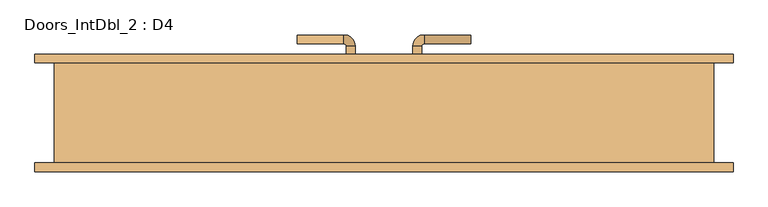
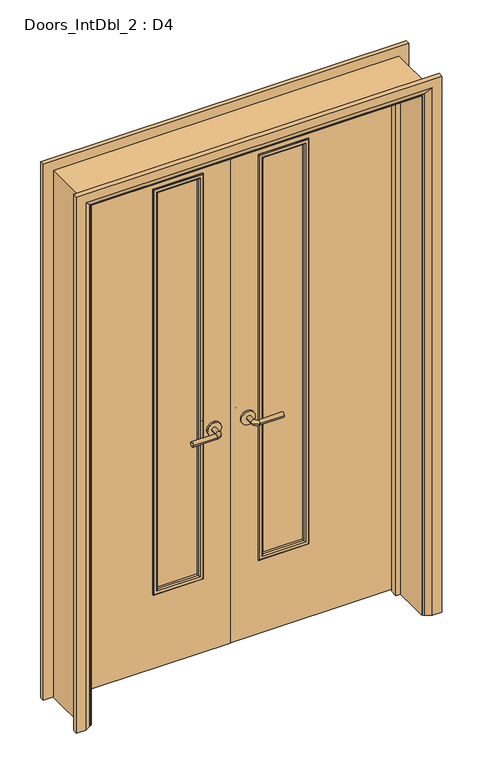
"""IFC4 building model written with IfcOpenShell, lengths in millimetres: door geometry, Doors_IntDbl_2 : D4."""

from ifc_helpers import new_model, si_unit, point, frame, frame_2d, origin, place, context, project, spatial, polyline, circle_curve, ellipse_curve, trimmed, segment, composite_curve, outline, extrude, faceted_brep, source, transform, mapped, element, save
from ifc_brep_helpers import plane_surface, cylinder_surface, revolved_surface, advanced_brep


def doors_intdbl_2_d4_7d0a9876(model_context):
    return source(origin(), model_context, "Body", "SolidModel", [
        advanced_brep(
        [(-65.0, 72.5, 1007.0), (-85.0, 72.5, 1007.0), (-65.0, 42.5, 1007.0), (-85.0, 42.5, 1007.0), (-90.0, 37.5, 1007.0), (-90.0, 17.5, 1007.0), (-195.0, 17.5, 1007.0), (-195.0, 37.5, 1007.0)],
        [
            (0, 1, circle_curve(frame((-75.0, 72.5, 1007.0), z_axis=(0.0, 1.0, 0.0), x_axis=(-1.0, 0.0, 0.0)), 10.0)),
            (1, 0, circle_curve(frame((-75.0, 72.5, 1007.0), z_axis=(0.0, 1.0, 0.0), x_axis=(-1.0, 0.0, 0.0)), 10.0)),
            (0, 2),
            (2, 3, circle_curve(frame((-75.0, 42.5, 1007.0), z_axis=(0.0, 1.0, 0.0), x_axis=(-1.0, 0.0, 0.0)), 10.0)),
            (3, 1),
            (3, 2, circle_curve(frame((-75.0, 42.5, 1007.0), z_axis=(0.0, 1.0, 0.0), x_axis=(-1.0, 0.0, 0.0)), 10.0)),
            (4, 3, circle_curve(frame((-90.0, 42.5, 1007.0), z_axis=(0.0, 0.0, 1.0), x_axis=(1.0, 0.0, 0.0)), 5.0)),
            (2, 5, circle_curve(frame((-90.0, 42.5, 1007.0), z_axis=(0.0, 0.0, -1.0), x_axis=(1.0, 0.0, 0.0)), 25.0)),
            (5, 4, circle_curve(frame((-90.0, 27.5, 1007.0), z_axis=(1.0, 0.0, 0.0), x_axis=(0.0, 1.0, 0.0)), 10.0)),
            (4, 5, circle_curve(frame((-90.0, 27.5, 1007.0), z_axis=(1.0, 0.0, 0.0), x_axis=(0.0, 1.0, 0.0)), 10.0)),
            (6, 7, circle_curve(frame((-195.0, 27.5, 1007.0), z_axis=(-1.0, 0.0, 0.0), x_axis=(0.0, 1.0, 0.0)), 10.0)),
            (7, 6, circle_curve(frame((-195.0, 27.5, 1007.0), z_axis=(-1.0, 0.0, 0.0), x_axis=(0.0, 1.0, 0.0)), 10.0)),
            (5, 6),
            (7, 4),
        ],
        [
            plane_surface(frame((-75.0, 72.5, 1007.0), z_axis=(0.0, 1.0, 0.0), x_axis=(0.0, 0.0, 1.0))),
            cylinder_surface(frame((-75.0, 72.5, 1007.0), z_axis=(0.0, 1.0, 0.0), x_axis=(-1.0, 0.0, 0.0)), 10.0),
            revolved_surface(trimmed(ellipse_curve(frame((-75.0, 42.5, 1007.0), z_axis=(0.0, 1.0, 0.0), x_axis=(-1.0, 0.0, 0.0)), 10.0, 10.0), [point((-65.0, 42.5, 1007.0))], [point((-85.0, 42.5, 1007.0))], True, "CARTESIAN"), (-90.0, 42.5, 1007.0), (0.0, 0.0, -1.0)),
            revolved_surface(trimmed(ellipse_curve(frame((-75.0, 42.5, 1007.0), z_axis=(0.0, 1.0, 0.0), x_axis=(-1.0, 0.0, 0.0)), 10.0, 10.0), [point((-85.0, 42.5, 1007.0))], [point((-65.0, 42.5, 1007.0))], True, "CARTESIAN"), (-90.0, 42.5, 1007.0), (0.0, 0.0, -1.0)),
            plane_surface(frame((-195.0, 27.5, 1007.0), z_axis=(-1.0, 0.0, 0.0), x_axis=(0.0, 0.0, 1.0))),
            cylinder_surface(frame((-90.0, 27.5, 1007.0), z_axis=(1.0, 0.0, 0.0), x_axis=(0.0, 1.0, 0.0)), 10.0),
        ],
        [
            (0, [[1, 2]]),
            (1, [[-1, 3, 4, 5]]),
            (1, [[-2, -5, 6, -3]]),
            (2, [[7, -4, 8, 9]]),
            (3, [[-8, -6, -7, 10]]),
            (4, [[11, 12]]),
            (5, [[-9, 13, -12, 14]]),
            (5, [[-10, -14, -11, -13]]),
        ],
    ),
        extrude(outline(composite_curve([segment(trimmed(circle_curve(frame_2d((1007.0, -72.5)), 30.0), [point((1007.0, -42.5))], [point((1007.0, -102.5))], False, "CARTESIAN"), True, "CONTINUOUS"), segment(trimmed(circle_curve(frame_2d((1007.0, -72.5)), 30.0), [point((1007.0, -102.5))], [point((1007.0, -42.5))], False, "CARTESIAN"), True, "CONTINUOUS")], self_intersect=False)), frame((0.0, 72.5, 0.0), z_axis=(0.0, 1.0, 0.0), x_axis=(0.0, 0.0, 1.0)), (0.0, 0.0, 1.0), 8.0),
        advanced_brep(
        [(-65.0, 120.5, 1007.0), (-85.0, 120.5, 1007.0), (-85.0, 150.5, 1007.0), (-65.0, 150.5, 1007.0), (-90.0, 155.5, 1007.0), (-90.0, 175.5, 1007.0), (-195.0, 175.5, 1007.0), (-195.0, 155.5, 1007.0)],
        [
            (0, 1, circle_curve(frame((-75.0, 120.5, 1007.0), z_axis=(0.0, -1.0, 0.0), x_axis=(-1.0, 0.0, 0.0)), 10.0)),
            (1, 0, circle_curve(frame((-75.0, 120.5, 1007.0), z_axis=(0.0, -1.0, 0.0), x_axis=(-1.0, 0.0, 0.0)), 10.0)),
            (1, 2),
            (2, 3, circle_curve(frame((-75.0, 150.5, 1007.0), z_axis=(0.0, -1.0, 0.0), x_axis=(-1.0, 0.0, 0.0)), 10.0)),
            (3, 0),
            (3, 2, circle_curve(frame((-75.0, 150.5, 1007.0), z_axis=(0.0, -1.0, 0.0), x_axis=(-1.0, 0.0, 0.0)), 10.0)),
            (4, 5, circle_curve(frame((-90.0, 165.5, 1007.0), z_axis=(1.0, 0.0, 0.0), x_axis=(0.0, -1.0, 0.0)), 10.0)),
            (5, 3, circle_curve(frame((-90.0, 150.5, 1007.0), z_axis=(0.0, 0.0, -1.0), x_axis=(1.0, 0.0, 0.0)), 25.0)),
            (2, 4, circle_curve(frame((-90.0, 150.5, 1007.0), z_axis=(0.0, 0.0, 1.0), x_axis=(1.0, 0.0, 0.0)), 5.0)),
            (5, 4, circle_curve(frame((-90.0, 165.5, 1007.0), z_axis=(1.0, 0.0, 0.0), x_axis=(0.0, -1.0, 0.0)), 10.0)),
            (6, 7, circle_curve(frame((-195.0, 165.5, 1007.0), z_axis=(-1.0, 0.0, 0.0), x_axis=(0.0, -1.0, 0.0)), 10.0)),
            (7, 6, circle_curve(frame((-195.0, 165.5, 1007.0), z_axis=(-1.0, 0.0, 0.0), x_axis=(0.0, -1.0, 0.0)), 10.0)),
            (4, 7),
            (6, 5),
        ],
        [
            plane_surface(frame((-75.0, 120.5, 1007.0), z_axis=(0.0, -1.0, 0.0), x_axis=(0.0, 0.0, 1.0))),
            cylinder_surface(frame((-75.0, 120.5, 1007.0), z_axis=(0.0, -1.0, 0.0), x_axis=(-1.0, 0.0, 0.0)), 10.0),
            revolved_surface(trimmed(ellipse_curve(frame((-75.0, 150.5, 1007.0), z_axis=(0.0, 1.0, 0.0), x_axis=(-1.0, 0.0, 0.0)), 10.0, 10.0), [point((-65.0, 150.5, 1007.0))], [point((-85.0, 150.5, 1007.0))], True, "CARTESIAN"), (-90.0, 150.5, 1007.0), (0.0, 0.0, -1.0)),
            revolved_surface(trimmed(ellipse_curve(frame((-75.0, 150.5, 1007.0), z_axis=(0.0, 1.0, 0.0), x_axis=(-1.0, 0.0, 0.0)), 10.0, 10.0), [point((-85.0, 150.5, 1007.0))], [point((-65.0, 150.5, 1007.0))], True, "CARTESIAN"), (-90.0, 150.5, 1007.0), (0.0, 0.0, -1.0)),
            plane_surface(frame((-195.0, 165.5, 1007.0), z_axis=(-1.0, 0.0, 0.0), x_axis=(0.0, 0.0, 1.0))),
            cylinder_surface(frame((-90.0, 165.5, 1007.0), z_axis=(1.0, 0.0, 0.0), x_axis=(0.0, -1.0, 0.0)), 10.0),
        ],
        [
            (0, [[1, 2]]),
            (1, [[3, 4, 5, -2]]),
            (1, [[-5, 6, -3, -1]]),
            (2, [[7, 8, -4, 9]]),
            (3, [[10, -9, -6, -8]]),
            (4, [[11, 12]]),
            (5, [[13, -11, 14, -7]]),
            (5, [[-14, -12, -13, -10]]),
        ],
    ),
        extrude(outline(composite_curve([segment(trimmed(circle_curve(frame_2d((1007.0, -72.5)), 30.0), [point((1007.0, -42.5))], [point((1007.0, -102.5))], False, "CARTESIAN"), True, "CONTINUOUS"), segment(trimmed(circle_curve(frame_2d((1007.0, -72.5)), 30.0), [point((1007.0, -102.5))], [point((1007.0, -42.5))], False, "CARTESIAN"), True, "CONTINUOUS")], self_intersect=False)), frame((0.0, 112.5, 0.0), z_axis=(0.0, 1.0, 0.0), x_axis=(0.0, 0.0, 1.0)), (0.0, 0.0, 1.0), 8.0),
        advanced_brep(
        [(65.0, 72.5, 1007.0), (85.0, 72.5, 1007.0), (85.0, 42.5, 1007.0), (65.0, 42.5, 1007.0), (90.0, 37.5, 1007.0), (90.0, 17.5, 1007.0), (195.0, 17.5, 1007.0), (195.0, 37.5, 1007.0)],
        [
            (0, 1, circle_curve(frame((75.0, 72.5, 1007.0), z_axis=(0.0, 1.0, 0.0), x_axis=(1.0, 0.0, 0.0)), 10.0)),
            (1, 0, circle_curve(frame((75.0, 72.5, 1007.0), z_axis=(0.0, 1.0, 0.0), x_axis=(1.0, 0.0, 0.0)), 10.0)),
            (1, 2),
            (2, 3, circle_curve(frame((75.0, 42.5, 1007.0), z_axis=(0.0, 1.0, 0.0), x_axis=(1.0, 0.0, 0.0)), 10.0)),
            (3, 0),
            (3, 2, circle_curve(frame((75.0, 42.5, 1007.0), z_axis=(0.0, 1.0, 0.0), x_axis=(1.0, 0.0, 0.0)), 10.0)),
            (4, 5, circle_curve(frame((90.0, 27.5, 1007.0), z_axis=(-1.0, 0.0, 0.0), x_axis=(0.0, 1.0, 0.0)), 10.0)),
            (5, 3, circle_curve(frame((90.0, 42.5, 1007.0), z_axis=(0.0, 0.0, -1.0), x_axis=(-1.0, 0.0, 0.0)), 25.0)),
            (2, 4, circle_curve(frame((90.0, 42.5, 1007.0), z_axis=(0.0, 0.0, 1.0), x_axis=(-1.0, 0.0, 0.0)), 5.0)),
            (5, 4, circle_curve(frame((90.0, 27.5, 1007.0), z_axis=(-1.0, 0.0, 0.0), x_axis=(0.0, 1.0, 0.0)), 10.0)),
            (6, 7, circle_curve(frame((195.0, 27.5, 1007.0), z_axis=(1.0, 0.0, 0.0), x_axis=(0.0, 1.0, 0.0)), 10.0)),
            (7, 6, circle_curve(frame((195.0, 27.5, 1007.0), z_axis=(1.0, 0.0, 0.0), x_axis=(0.0, 1.0, 0.0)), 10.0)),
            (4, 7),
            (6, 5),
        ],
        [
            plane_surface(frame((75.0, 72.5, 1007.0), z_axis=(0.0, 1.0, 0.0), x_axis=(0.0, 0.0, 1.0))),
            cylinder_surface(frame((75.0, 72.5, 1007.0), z_axis=(0.0, 1.0, 0.0), x_axis=(1.0, 0.0, 0.0)), 10.0),
            revolved_surface(trimmed(ellipse_curve(frame((75.0, 42.5, 1007.0), z_axis=(0.0, -1.0, 0.0), x_axis=(1.0, 0.0, 0.0)), 10.0, 10.0), [point((65.0, 42.5, 1007.0))], [point((85.0, 42.5, 1007.0))], True, "CARTESIAN"), (90.0, 42.5, 1007.0), (0.0, 0.0, -1.0)),
            revolved_surface(trimmed(ellipse_curve(frame((75.0, 42.5, 1007.0), z_axis=(0.0, -1.0, 0.0), x_axis=(1.0, 0.0, 0.0)), 10.0, 10.0), [point((85.0, 42.5, 1007.0))], [point((65.0, 42.5, 1007.0))], True, "CARTESIAN"), (90.0, 42.5, 1007.0), (0.0, 0.0, -1.0)),
            plane_surface(frame((195.0, 27.5, 1007.0), z_axis=(1.0, 0.0, 0.0), x_axis=(0.0, 0.0, 1.0))),
            cylinder_surface(frame((90.0, 27.5, 1007.0), z_axis=(-1.0, 0.0, 0.0), x_axis=(0.0, 1.0, 0.0)), 10.0),
        ],
        [
            (0, [[1, 2]]),
            (1, [[3, 4, 5, -2]]),
            (1, [[-5, 6, -3, -1]]),
            (2, [[7, 8, -4, 9]]),
            (3, [[10, -9, -6, -8]]),
            (4, [[11, 12]]),
            (5, [[13, -11, 14, -7]]),
            (5, [[-14, -12, -13, -10]]),
        ],
    ),
        extrude(outline(composite_curve([segment(trimmed(circle_curve(frame_2d((1007.0, 72.5)), 30.0), [point((1007.0, 42.5))], [point((1007.0, 102.5))], False, "CARTESIAN"), True, "CONTINUOUS"), segment(trimmed(circle_curve(frame_2d((1007.0, 72.5)), 30.0), [point((1007.0, 102.5))], [point((1007.0, 42.5))], False, "CARTESIAN"), True, "CONTINUOUS")], self_intersect=False)), frame((0.0, 72.5, 0.0), z_axis=(0.0, 1.0, 0.0), x_axis=(0.0, 0.0, 1.0)), (0.0, 0.0, 1.0), 8.0),
        advanced_brep(
        [(65.0, 120.5, 1007.0), (85.0, 120.5, 1007.0), (65.0, 150.5, 1007.0), (85.0, 150.5, 1007.0), (90.0, 155.5, 1007.0), (90.0, 175.5, 1007.0), (195.0, 175.5, 1007.0), (195.0, 155.5, 1007.0)],
        [
            (0, 1, circle_curve(frame((75.0, 120.5, 1007.0), z_axis=(0.0, -1.0, 0.0), x_axis=(1.0, 0.0, 0.0)), 10.0)),
            (1, 0, circle_curve(frame((75.0, 120.5, 1007.0), z_axis=(0.0, -1.0, 0.0), x_axis=(1.0, 0.0, 0.0)), 10.0)),
            (0, 2),
            (2, 3, circle_curve(frame((75.0, 150.5, 1007.0), z_axis=(0.0, -1.0, 0.0), x_axis=(1.0, 0.0, 0.0)), 10.0)),
            (3, 1),
            (3, 2, circle_curve(frame((75.0, 150.5, 1007.0), z_axis=(0.0, -1.0, 0.0), x_axis=(1.0, 0.0, 0.0)), 10.0)),
            (4, 3, circle_curve(frame((90.0, 150.5, 1007.0), z_axis=(0.0, 0.0, 1.0), x_axis=(-1.0, 0.0, 0.0)), 5.0)),
            (2, 5, circle_curve(frame((90.0, 150.5, 1007.0), z_axis=(0.0, 0.0, -1.0), x_axis=(-1.0, 0.0, 0.0)), 25.0)),
            (5, 4, circle_curve(frame((90.0, 165.5, 1007.0), z_axis=(-1.0, 0.0, 0.0), x_axis=(0.0, -1.0, 0.0)), 10.0)),
            (4, 5, circle_curve(frame((90.0, 165.5, 1007.0), z_axis=(-1.0, 0.0, 0.0), x_axis=(0.0, -1.0, 0.0)), 10.0)),
            (6, 7, circle_curve(frame((195.0, 165.5, 1007.0), z_axis=(1.0, 0.0, 0.0), x_axis=(0.0, -1.0, 0.0)), 10.0)),
            (7, 6, circle_curve(frame((195.0, 165.5, 1007.0), z_axis=(1.0, 0.0, 0.0), x_axis=(0.0, -1.0, 0.0)), 10.0)),
            (5, 6),
            (7, 4),
        ],
        [
            plane_surface(frame((75.0, 120.5, 1007.0), z_axis=(0.0, -1.0, 0.0), x_axis=(0.0, 0.0, 1.0))),
            cylinder_surface(frame((75.0, 120.5, 1007.0), z_axis=(0.0, -1.0, 0.0), x_axis=(1.0, 0.0, 0.0)), 10.0),
            revolved_surface(trimmed(ellipse_curve(frame((75.0, 150.5, 1007.0), z_axis=(0.0, -1.0, 0.0), x_axis=(1.0, 0.0, 0.0)), 10.0, 10.0), [point((65.0, 150.5, 1007.0))], [point((85.0, 150.5, 1007.0))], True, "CARTESIAN"), (90.0, 150.5, 1007.0), (0.0, 0.0, -1.0)),
            revolved_surface(trimmed(ellipse_curve(frame((75.0, 150.5, 1007.0), z_axis=(0.0, -1.0, 0.0), x_axis=(1.0, 0.0, 0.0)), 10.0, 10.0), [point((85.0, 150.5, 1007.0))], [point((65.0, 150.5, 1007.0))], True, "CARTESIAN"), (90.0, 150.5, 1007.0), (0.0, 0.0, -1.0)),
            plane_surface(frame((195.0, 165.5, 1007.0), z_axis=(1.0, 0.0, 0.0), x_axis=(0.0, 0.0, 1.0))),
            cylinder_surface(frame((90.0, 165.5, 1007.0), z_axis=(-1.0, 0.0, 0.0), x_axis=(0.0, -1.0, 0.0)), 10.0),
        ],
        [
            (0, [[1, 2]]),
            (1, [[-1, 3, 4, 5]]),
            (1, [[-2, -5, 6, -3]]),
            (2, [[7, -4, 8, 9]]),
            (3, [[-8, -6, -7, 10]]),
            (4, [[11, 12]]),
            (5, [[-9, 13, -12, 14]]),
            (5, [[-10, -14, -11, -13]]),
        ],
    ),
        extrude(outline(composite_curve([segment(trimmed(circle_curve(frame_2d((1007.0, 72.5)), 30.0), [point((1007.0, 42.5))], [point((1007.0, 102.5))], False, "CARTESIAN"), True, "CONTINUOUS"), segment(trimmed(circle_curve(frame_2d((1007.0, 72.5)), 30.0), [point((1007.0, 102.5))], [point((1007.0, 42.5))], False, "CARTESIAN"), True, "CONTINUOUS")], self_intersect=False)), frame((0.0, 112.5, 0.0), z_axis=(0.0, 1.0, 0.0), x_axis=(0.0, 0.0, 1.0)), (0.0, 0.0, 1.0), 8.0),
        extrude(outline(polyline([(2392.0, -742.0), (0.0, -742.0), (0.0, -710.0), (2360.0, -710.0), (2360.0, 710.0), (0.0, 710.0), (0.0, 742.0), (2392.0, 742.0), (2392.0, -742.0)])), frame((0.0, -112.5, 0.0), z_axis=(0.0, 1.0, 0.0), x_axis=(0.0, 0.0, 1.0)), (0.0, 0.0, 1.0), 225.0),
        faceted_brep([(-691.0, 77.5, 0.0), (-691.0, 45.5, 0.0), (-710.0, 45.5, 0.0), (-710.0, 77.5, 0.0), (-691.0, 77.5, 2341.0), (-691.0, 45.5, 2341.0), (-710.0, 45.5, 2360.0), (-710.0, 77.5, 2360.0), (691.0, 77.5, 0.0), (710.0, 77.5, 0.0), (710.0, 45.5, 0.0), (691.0, 45.5, 0.0), (691.0, 77.5, 2341.0), (710.0, 77.5, 2360.0), (710.0, 45.5, 2360.0), (691.0, 45.5, 2341.0)], [[[0, 1, 2, 3]], [[1, 0, 4, 5]], [[2, 1, 5, 6]], [[3, 2, 6, 7]], [[0, 3, 7, 4]], [[8, 9, 10, 11]], [[12, 13, 9, 8]], [[13, 14, 10, 9]], [[14, 15, 11, 10]], [[15, 12, 8, 11]], [[5, 4, 12, 15]], [[6, 5, 15, 14]], [[7, 6, 14, 13]], [[4, 7, 13, 12]]]),
        advanced_brep(
        [(785.0, 132.5, 0.0), (785.0, 112.5, 0.0), (715.0, 112.5, 0.0), (719.0, 118.5, 0.0), (745.0, 132.5, 0.0), (785.0, 132.5, 2435.0), (785.0, 112.5, 2435.0), (-785.0, 112.5, 2435.0), (-785.0, 112.5, 0.0), (-715.0, 112.5, 0.0), (-715.0, 112.5, 2365.0), (715.0, 112.5, 2365.0), (719.0, 118.5, 2369.0), (745.0, 132.5, 2395.0), (-745.0, 132.5, 2395.0), (-745.0, 132.5, 0.0), (-785.0, 132.5, 0.0), (-785.0, 132.5, 2435.0), (-719.0, 118.5, 0.0), (-719.0, 118.5, 2369.0)],
        [
            (0, 1),
            (1, 2),
            (2, 3, circle_curve(frame((723.0, 111.5, 0.0), z_axis=(0.0, 0.0, -1.0), x_axis=(1.0, 0.0, 0.0)), 8.0622577)),
            (3, 4),
            (4, 0),
            (0, 5),
            (5, 6),
            (6, 1),
            (6, 7),
            (7, 8),
            (8, 9),
            (9, 10),
            (10, 11),
            (11, 2),
            (11, 12, ellipse_curve(frame((723.0, 111.5, 2373.0), z_axis=(0.7071067811865475, 0.0, -0.7071067811865475), x_axis=(-0.7071067811865474, 0.0, -0.7071067811865476)), 11.4017543, 8.0622577)),
            (12, 3),
            (12, 13),
            (13, 4),
            (13, 14),
            (14, 15),
            (15, 16),
            (16, 17),
            (17, 5),
            (7, 17),
            (16, 8),
            (15, 18),
            (18, 9, circle_curve(frame((-723.0, 111.5, 0.0), z_axis=(0.0, 0.0, -1.0), x_axis=(-1.0, 0.0, 0.0)), 8.0622577)),
            (19, 10, ellipse_curve(frame((-723.0, 111.5, 2373.0), z_axis=(-0.7071067811865475, 0.0, -0.7071067811865475), x_axis=(-0.7071067811865474, 0.0, 0.7071067811865476)), 11.4017543, 8.0622577)),
            (18, 19),
            (14, 19),
            (19, 12),
        ],
        [
            plane_surface(frame((715.0, 112.5, 0.0), z_axis=(0.0, 0.0, -1.0), x_axis=(0.0, -1.0, 0.0))),
            plane_surface(frame((785.0, 132.5, 0.0), z_axis=(1.0, 0.0, 0.0), x_axis=(0.0, 0.0, 1.0))),
            plane_surface(frame((785.0, 112.5, 0.0), z_axis=(0.0, -1.0, 0.0), x_axis=(0.0, 0.0, 1.0))),
            cylinder_surface(frame((723.0, 111.5, 0.0), z_axis=(0.0, 0.0, -1.0), x_axis=(1.0, 0.0, 0.0)), 8.0622577),
            plane_surface(frame((719.0, 118.5, 0.0), z_axis=(-0.4740998230350126, 0.8804710999221779, 0.0), x_axis=(0.0, 0.0, 1.0))),
            plane_surface(frame((745.0, 132.5, 0.0), z_axis=(0.0, 1.0, 0.0), x_axis=(0.0, 0.0, 1.0))),
            plane_surface(frame((-785.0, 132.5, 2435.0), z_axis=(-1.0, 0.0, 0.0), x_axis=(0.0, 0.0, -1.0))),
            plane_surface(frame((-715.0, 112.5, 0.0), z_axis=(0.0, 0.0, -1.0), x_axis=(0.0, -1.0, 0.0))),
            cylinder_surface(frame((-723.0, 111.5, 2365.0), z_axis=(0.0, 0.0, 1.0), x_axis=(-1.0, 0.0, 0.0)), 8.0622577),
            plane_surface(frame((-719.0, 118.5, 2369.0), z_axis=(0.4740998230350183, 0.8804710999221749, 0.0), x_axis=(0.0, 0.0, -1.0))),
            plane_surface(frame((785.0, 132.5, 2435.0), z_axis=(0.0, 0.0, 1.0), x_axis=(-1.0, 0.0, 0.0))),
            cylinder_surface(frame((715.0, 111.5, 2373.0), z_axis=(1.0, 0.0, 0.0), x_axis=(0.0, 0.0, 1.0)), 8.0622577),
            plane_surface(frame((719.0, 118.5, 2369.0), z_axis=(0.0, 0.8804710999221763, -0.4740998230350154), x_axis=(-1.0, 0.0, 0.0))),
        ],
        [
            (0, [[1, 2, 3, 4, 5]]),
            (1, [[-1, 6, 7, 8]]),
            (2, [[-2, -8, 9, 10, 11, 12, 13, 14]]),
            (3, [[-3, -14, 15, 16]]),
            (4, [[-4, -16, 17, 18]]),
            (5, [[-5, -18, 19, 20, 21, 22, 23, -6]]),
            (6, [[24, -22, 25, -10]]),
            (7, [[-21, 26, 27, -11, -25]]),
            (8, [[28, -12, -27, 29]]),
            (9, [[30, -29, -26, -20]]),
            (10, [[-7, -23, -24, -9]]),
            (11, [[-15, -13, -28, 31]]),
            (12, [[-17, -31, -30, -19]]),
        ],
    ),
        advanced_brep(
        [(-785.0, -132.5, 0.0), (-785.0, -112.5, 0.0), (-715.0, -112.5, 0.0), (-719.0, -118.5, 0.0), (-745.0, -132.5, 0.0), (-785.0, -132.5, 2435.0), (-785.0, -112.5, 2435.0), (785.0, -112.5, 2435.0), (785.0, -112.5, 0.0), (715.0, -112.5, 0.0), (715.0, -112.5, 2365.0), (-715.0, -112.5, 2365.0), (-719.0, -118.5, 2369.0), (-745.0, -132.5, 2395.0), (745.0, -132.5, 2395.0), (745.0, -132.5, 0.0), (785.0, -132.5, 0.0), (785.0, -132.5, 2435.0), (719.0, -118.5, 0.0), (719.0, -118.5, 2369.0)],
        [
            (0, 1),
            (1, 2),
            (2, 3, circle_curve(frame((-723.0, -111.5, 0.0), z_axis=(0.0, 0.0, -1.0), x_axis=(-1.0, 0.0, 0.0)), 8.0622577)),
            (3, 4),
            (4, 0),
            (0, 5),
            (5, 6),
            (6, 1),
            (6, 7),
            (7, 8),
            (8, 9),
            (9, 10),
            (10, 11),
            (11, 2),
            (11, 12, ellipse_curve(frame((-723.0, -111.5, 2373.0), z_axis=(-0.7071067811865475, 0.0, -0.7071067811865475), x_axis=(0.7071067811865474, 0.0, -0.7071067811865476)), 11.4017543, 8.0622577)),
            (12, 3),
            (12, 13),
            (13, 4),
            (13, 14),
            (14, 15),
            (15, 16),
            (16, 17),
            (17, 5),
            (7, 17),
            (16, 8),
            (15, 18),
            (18, 9, circle_curve(frame((723.0, -111.5, 0.0), z_axis=(0.0, 0.0, -1.0), x_axis=(1.0, 0.0, 0.0)), 8.0622577)),
            (19, 10, ellipse_curve(frame((723.0, -111.5, 2373.0), z_axis=(0.7071067811865475, 0.0, -0.7071067811865475), x_axis=(0.7071067811865474, 0.0, 0.7071067811865476)), 11.4017543, 8.0622577)),
            (18, 19),
            (14, 19),
            (19, 12),
        ],
        [
            plane_surface(frame((-715.0, -112.5, 0.0), z_axis=(0.0, 0.0, -1.0), x_axis=(0.0, -1.0, 0.0))),
            plane_surface(frame((-785.0, -132.5, 0.0), z_axis=(-1.0, 0.0, 0.0), x_axis=(0.0, 0.0, 1.0))),
            plane_surface(frame((-785.0, -112.5, 0.0), z_axis=(0.0, 1.0, 0.0), x_axis=(0.0, 0.0, 1.0))),
            cylinder_surface(frame((-723.0, -111.5, 0.0), z_axis=(0.0, 0.0, -1.0), x_axis=(-1.0, 0.0, 0.0)), 8.0622577),
            plane_surface(frame((-719.0, -118.5, 0.0), z_axis=(0.4740998230350183, -0.8804710999221749, 0.0), x_axis=(0.0, 0.0, 1.0))),
            plane_surface(frame((-745.0, -132.5, 0.0), z_axis=(0.0, -1.0, 0.0), x_axis=(0.0, 0.0, 1.0))),
            plane_surface(frame((785.0, -132.5, 2435.0), z_axis=(1.0, 0.0, 0.0), x_axis=(0.0, 0.0, -1.0))),
            plane_surface(frame((715.0, -112.5, 0.0), z_axis=(0.0, 0.0, -1.0), x_axis=(0.0, -1.0, 0.0))),
            cylinder_surface(frame((723.0, -111.5, 2365.0), z_axis=(0.0, 0.0, 1.0), x_axis=(1.0, 0.0, 0.0)), 8.0622577),
            plane_surface(frame((719.0, -118.5, 2369.0), z_axis=(-0.4740998230350183, -0.8804710999221749, 0.0), x_axis=(0.0, 0.0, -1.0))),
            plane_surface(frame((-785.0, -132.5, 2435.0), z_axis=(0.0, 0.0, 1.0), x_axis=(1.0, 0.0, 0.0))),
            cylinder_surface(frame((-715.0, -111.5, 2373.0), z_axis=(-1.0, 0.0, 0.0), x_axis=(0.0, 0.0, 1.0)), 8.0622577),
            plane_surface(frame((-719.0, -118.5, 2369.0), z_axis=(0.0, -0.8804710999221749, -0.4740998230350183), x_axis=(1.0, 0.0, 0.0))),
        ],
        [
            (0, [[1, 2, 3, 4, 5]]),
            (1, [[-1, 6, 7, 8]]),
            (2, [[-2, -8, 9, 10, 11, 12, 13, 14]]),
            (3, [[-3, -14, 15, 16]]),
            (4, [[-4, -16, 17, 18]]),
            (5, [[-5, -18, 19, 20, 21, 22, 23, -6]]),
            (6, [[24, -22, 25, -10]]),
            (7, [[-21, 26, 27, -11, -25]]),
            (8, [[28, -12, -27, 29]]),
            (9, [[30, -29, -26, -20]]),
            (10, [[-7, -23, -24, -9]]),
            (11, [[-15, -13, -28, 31]]),
            (12, [[-17, -31, -30, -19]]),
        ],
    ),
        extrude(outline(polyline([(5.753223, 707.0), (2357.0, 707.0), (2357.0, 1.5), (5.753223, 1.5), (5.753223, 707.0)]), holes=[polyline([(2175.0, 126.5), (2175.0, 326.5), (350.0, 326.5), (350.0, 126.5), (2175.0, 126.5)])]), frame((0.0, 80.5, 0.0), z_axis=(0.0, 1.0, 0.0), x_axis=(0.0, 0.0, 1.0)), (0.0, 0.0, 1.0), 32.0),
        extrude(outline(polyline([(5.753223, -707.0), (5.753223, -1.5), (2357.0, -1.5), (2357.0, -707.0), (5.753223, -707.0)]), holes=[polyline([(2175.0, -326.5), (2175.0, -126.5), (350.0, -126.5), (350.0, -326.5), (2175.0, -326.5)])]), frame((0.0, 80.5, 0.0), z_axis=(0.0, 1.0, 0.0), x_axis=(0.0, 0.0, 1.0)), (0.0, 0.0, 1.0), 32.0),
        extrude(outline(polyline([(326.5, 90.5), (126.5, 90.5), (126.5, 102.5), (326.5, 102.5), (326.5, 90.5)])), frame((0.0, 0.0, 350.0), z_axis=(0.0, 0.0, 1.0), x_axis=(1.0, 0.0, 0.0)), (0.0, 0.0, 1.0), 1825.0),
        extrude(outline(polyline([(-126.5, 90.5), (-326.5, 90.5), (-326.5, 102.5), (-126.5, 102.5), (-126.5, 90.5)])), frame((0.0, 0.0, 350.0), z_axis=(0.0, 0.0, 1.0), x_axis=(1.0, 0.0, 0.0)), (0.0, 0.0, 1.0), 1825.0),
        advanced_brep(
        [(-326.5, 102.5, 2175.0), (-326.5, 112.5, 2175.0), (-326.5, 112.5, 350.0), (-326.5, 102.5, 350.0), (-314.5, 113.5, 2163.0), (-314.5, 102.5, 2163.0), (-314.5, 102.5, 362.0), (-314.5, 113.5, 362.0), (-319.5, 118.5, 2168.0), (-319.5, 118.5, 357.0), (-334.5, 116.5, 2183.0), (-332.5, 118.5, 2181.0), (-332.5, 118.5, 344.0), (-334.5, 116.5, 342.0), (-334.5, 112.5, 2183.0), (-334.5, 112.5, 342.0), (-126.5, 112.5, 350.0), (-126.5, 102.5, 350.0), (-138.5, 102.5, 362.0), (-138.5, 113.5, 362.0), (-133.5, 118.5, 357.0), (-120.5, 118.5, 344.0), (-118.5, 116.5, 342.0), (-118.5, 112.5, 342.0), (-126.5, 112.5, 2175.0), (-126.5, 102.5, 2175.0), (-138.5, 102.5, 2163.0), (-138.5, 113.5, 2163.0), (-133.5, 118.5, 2168.0), (-120.5, 118.5, 2181.0), (-118.5, 116.5, 2183.0), (-118.5, 112.5, 2183.0)],
        [
            (0, 1),
            (1, 2),
            (2, 3),
            (3, 0),
            (4, 5),
            (5, 6),
            (6, 7),
            (7, 4),
            (8, 4, ellipse_curve(frame((-319.5, 113.5, 2168.0), z_axis=(-0.7071067811865475, 0.0, -0.7071067811865475), x_axis=(-0.7071067811865474, 0.0, 0.7071067811865476)), 7.0710678, 5.0)),
            (7, 9, ellipse_curve(frame((-319.5, 113.5, 357.0), z_axis=(-0.7071067811865475, 0.0, 0.7071067811865475), x_axis=(0.7071067811865474, 0.0, 0.7071067811865476)), 7.0710678, 5.0)),
            (9, 8),
            (10, 11, ellipse_curve(frame((-332.5, 116.5, 2181.0), z_axis=(-0.7071067811865475, 0.0, -0.7071067811865475), x_axis=(-0.7071067811865474, 0.0, 0.7071067811865476)), 2.8284271, 2.0)),
            (11, 12),
            (12, 13, ellipse_curve(frame((-332.5, 116.5, 344.0), z_axis=(-0.7071067811865475, 0.0, 0.7071067811865475), x_axis=(0.7071067811865474, 0.0, 0.7071067811865476)), 2.8284271, 2.0)),
            (13, 10),
            (14, 10),
            (13, 15),
            (15, 14),
            (2, 16),
            (16, 17),
            (17, 3),
            (6, 18),
            (18, 19),
            (19, 7),
            (19, 20, ellipse_curve(frame((-133.5, 113.5, 357.0), z_axis=(-0.7071067811865475, 0.0, -0.7071067811865475), x_axis=(-0.7071067811865476, 0.0, 0.7071067811865474)), 7.0710678, 5.0)),
            (20, 9),
            (12, 21),
            (21, 22, ellipse_curve(frame((-120.5, 116.5, 344.0), z_axis=(-0.7071067811865475, 0.0, -0.7071067811865475), x_axis=(-0.7071067811865476, 0.0, 0.7071067811865474)), 2.8284271, 2.0)),
            (22, 13),
            (22, 23),
            (23, 15),
            (16, 24),
            (24, 25),
            (25, 17),
            (18, 26),
            (26, 27),
            (27, 19),
            (27, 28, ellipse_curve(frame((-133.5, 113.5, 2168.0), z_axis=(0.7071067811865475, 0.0, -0.7071067811865475), x_axis=(-0.7071067811865474, 0.0, -0.7071067811865476)), 7.0710678, 5.0)),
            (28, 20),
            (21, 29),
            (29, 30, ellipse_curve(frame((-120.5, 116.5, 2181.0), z_axis=(0.7071067811865475, 0.0, -0.7071067811865475), x_axis=(-0.7071067811865474, 0.0, -0.7071067811865476)), 2.8284271, 2.0)),
            (30, 22),
            (30, 31),
            (31, 23),
            (31, 14),
            (1, 24),
            (0, 25),
            (5, 26),
            (4, 27),
            (8, 28),
            (11, 29),
            (10, 30),
        ],
        [
            plane_surface(frame((-326.5, 112.5, 2175.0), z_axis=(-1.0, 0.0, 0.0), x_axis=(0.0, 0.0, -1.0))),
            plane_surface(frame((-314.5, 102.5, 2163.0), z_axis=(1.0, 0.0, 0.0), x_axis=(0.0, 0.0, -1.0))),
            cylinder_surface(frame((-319.5, 113.5, 2175.0), z_axis=(0.0, 0.0, 1.0), x_axis=(-1.0, 0.0, 0.0)), 5.0),
            cylinder_surface(frame((-332.5, 116.5, 2175.0), z_axis=(0.0, 0.0, 1.0), x_axis=(-1.0, 0.0, 0.0)), 2.0),
            plane_surface(frame((-334.5, 116.5, 2183.0), z_axis=(-1.0, 0.0, 0.0), x_axis=(0.0, 0.0, -1.0))),
            plane_surface(frame((-326.5, 112.5, 350.0), z_axis=(0.0, 0.0, -1.0), x_axis=(1.0, 0.0, 0.0))),
            plane_surface(frame((-314.5, 102.5, 362.0), z_axis=(0.0, 0.0, 1.0), x_axis=(1.0, 0.0, 0.0))),
            cylinder_surface(frame((-326.5, 113.5, 357.0), z_axis=(-1.0, 0.0, 0.0), x_axis=(0.0, 0.0, -1.0)), 5.0),
            cylinder_surface(frame((-326.5, 116.5, 344.0), z_axis=(-1.0, 0.0, 0.0), x_axis=(0.0, 0.0, -1.0)), 2.0),
            plane_surface(frame((-334.5, 116.5, 342.0), z_axis=(0.0, 0.0, -1.0), x_axis=(1.0, 0.0, 0.0))),
            plane_surface(frame((-126.5, 112.5, 350.0), z_axis=(1.0, 0.0, 0.0), x_axis=(0.0, 0.0, 1.0))),
            plane_surface(frame((-138.5, 102.5, 362.0), z_axis=(-1.0, 0.0, 0.0), x_axis=(0.0, 0.0, 1.0))),
            cylinder_surface(frame((-133.5, 113.5, 350.0), z_axis=(0.0, 0.0, -1.0), x_axis=(1.0, 0.0, 0.0)), 5.0),
            cylinder_surface(frame((-120.5, 116.5, 350.0), z_axis=(0.0, 0.0, -1.0), x_axis=(1.0, 0.0, 0.0)), 2.0),
            plane_surface(frame((-118.5, 116.5, 342.0), z_axis=(1.0, 0.0, 0.0), x_axis=(0.0, 0.0, 1.0))),
            plane_surface(frame((-118.5, 112.5, 2183.0), z_axis=(0.0, -1.0, 0.0), x_axis=(-1.0, 0.0, 0.0))),
            plane_surface(frame((-126.5, 112.5, 2175.0), z_axis=(0.0, 0.0, 1.0), x_axis=(-1.0, 0.0, 0.0))),
            plane_surface(frame((-126.5, 102.5, 2175.0), z_axis=(0.0, -1.0, 0.0), x_axis=(-1.0, 0.0, 0.0))),
            plane_surface(frame((-138.5, 102.5, 2163.0), z_axis=(0.0, 0.0, -1.0), x_axis=(-1.0, 0.0, 0.0))),
            cylinder_surface(frame((-126.5, 113.5, 2168.0), z_axis=(1.0, 0.0, 0.0), x_axis=(0.0, 0.0, 1.0)), 5.0),
            plane_surface(frame((-133.5, 118.5, 2168.0), z_axis=(0.0, 1.0, 0.0), x_axis=(-1.0, 0.0, 0.0))),
            cylinder_surface(frame((-126.5, 116.5, 2181.0), z_axis=(1.0, 0.0, 0.0), x_axis=(0.0, 0.0, 1.0)), 2.0),
            plane_surface(frame((-118.5, 116.5, 2183.0), z_axis=(0.0, 0.0, 1.0), x_axis=(-1.0, 0.0, 0.0))),
        ],
        [
            (0, [[1, 2, 3, 4]]),
            (1, [[5, 6, 7, 8]]),
            (2, [[9, -8, 10, 11]]),
            (3, [[12, 13, 14, 15]]),
            (4, [[16, -15, 17, 18]]),
            (5, [[-3, 19, 20, 21]]),
            (6, [[-7, 22, 23, 24]]),
            (7, [[-10, -24, 25, 26]]),
            (8, [[-14, 27, 28, 29]]),
            (9, [[-17, -29, 30, 31]]),
            (10, [[-20, 32, 33, 34]]),
            (11, [[-23, 35, 36, 37]]),
            (12, [[-25, -37, 38, 39]]),
            (13, [[-28, 40, 41, 42]]),
            (14, [[-30, -42, 43, 44]]),
            (15, [[-31, -44, 45, -18], [46, -32, -19, -2]]),
            (16, [[-33, -46, -1, 47]]),
            (17, [[-21, -34, -47, -4], [48, -35, -22, -6]]),
            (18, [[-36, -48, -5, 49]]),
            (19, [[-38, -49, -9, 50]]),
            (20, [[51, -40, -27, -13], [-26, -39, -50, -11]]),
            (21, [[-41, -51, -12, 52]]),
            (22, [[-43, -52, -16, -45]]),
        ],
    ),
        advanced_brep(
        [(326.5, 102.5, 350.0), (326.5, 112.5, 350.0), (326.5, 112.5, 2175.0), (326.5, 102.5, 2175.0), (314.5, 113.5, 362.0), (314.5, 102.5, 362.0), (314.5, 102.5, 2163.0), (314.5, 113.5, 2163.0), (319.5, 118.5, 357.0), (319.5, 118.5, 2168.0), (334.5, 116.5, 342.0), (332.5, 118.5, 344.0), (332.5, 118.5, 2181.0), (334.5, 116.5, 2183.0), (334.5, 112.5, 342.0), (334.5, 112.5, 2183.0), (126.5, 112.5, 2175.0), (126.5, 102.5, 2175.0), (138.5, 102.5, 2163.0), (138.5, 113.5, 2163.0), (133.5, 118.5, 2168.0), (120.5, 118.5, 2181.0), (118.5, 116.5, 2183.0), (118.5, 112.5, 2183.0), (126.5, 112.5, 350.0), (126.5, 102.5, 350.0), (138.5, 102.5, 362.0), (138.5, 113.5, 362.0), (133.5, 118.5, 357.0), (120.5, 118.5, 344.0), (118.5, 116.5, 342.0), (118.5, 112.5, 342.0)],
        [
            (0, 1),
            (1, 2),
            (2, 3),
            (3, 0),
            (4, 5),
            (5, 6),
            (6, 7),
            (7, 4),
            (8, 4, ellipse_curve(frame((319.5, 113.5, 357.0), z_axis=(0.7071067811865475, 0.0, 0.7071067811865475), x_axis=(0.7071067811865474, 0.0, -0.7071067811865476)), 7.0710678, 5.0)),
            (7, 9, ellipse_curve(frame((319.5, 113.5, 2168.0), z_axis=(0.7071067811865475, 0.0, -0.7071067811865475), x_axis=(-0.7071067811865474, 0.0, -0.7071067811865476)), 7.0710678, 5.0)),
            (9, 8),
            (10, 11, ellipse_curve(frame((332.5, 116.5, 344.0), z_axis=(0.7071067811865475, 0.0, 0.7071067811865475), x_axis=(0.7071067811865474, 0.0, -0.7071067811865476)), 2.8284271, 2.0)),
            (11, 12),
            (12, 13, ellipse_curve(frame((332.5, 116.5, 2181.0), z_axis=(0.7071067811865475, 0.0, -0.7071067811865475), x_axis=(-0.7071067811865474, 0.0, -0.7071067811865476)), 2.8284271, 2.0)),
            (13, 10),
            (14, 10),
            (13, 15),
            (15, 14),
            (2, 16),
            (16, 17),
            (17, 3),
            (6, 18),
            (18, 19),
            (19, 7),
            (19, 20, ellipse_curve(frame((133.5, 113.5, 2168.0), z_axis=(0.7071067811865475, 0.0, 0.7071067811865475), x_axis=(0.7071067811865476, 0.0, -0.7071067811865474)), 7.0710678, 5.0)),
            (20, 9),
            (12, 21),
            (21, 22, ellipse_curve(frame((120.5, 116.5, 2181.0), z_axis=(0.7071067811865475, 0.0, 0.7071067811865475), x_axis=(0.7071067811865476, 0.0, -0.7071067811865474)), 2.8284271, 2.0)),
            (22, 13),
            (22, 23),
            (23, 15),
            (16, 24),
            (24, 25),
            (25, 17),
            (18, 26),
            (26, 27),
            (27, 19),
            (27, 28, ellipse_curve(frame((133.5, 113.5, 357.0), z_axis=(-0.7071067811865475, 0.0, 0.7071067811865475), x_axis=(0.7071067811865474, 0.0, 0.7071067811865476)), 7.0710678, 5.0)),
            (28, 20),
            (21, 29),
            (29, 30, ellipse_curve(frame((120.5, 116.5, 344.0), z_axis=(-0.7071067811865475, 0.0, 0.7071067811865475), x_axis=(0.7071067811865474, 0.0, 0.7071067811865476)), 2.8284271, 2.0)),
            (30, 22),
            (30, 31),
            (31, 23),
            (31, 14),
            (1, 24),
            (0, 25),
            (5, 26),
            (4, 27),
            (8, 28),
            (11, 29),
            (10, 30),
        ],
        [
            plane_surface(frame((326.5, 112.5, 350.0), z_axis=(1.0, 0.0, 0.0), x_axis=(0.0, 0.0, 1.0))),
            plane_surface(frame((314.5, 102.5, 362.0), z_axis=(-1.0, 0.0, 0.0), x_axis=(0.0, 0.0, 1.0))),
            cylinder_surface(frame((319.5, 113.5, 350.0), z_axis=(0.0, 0.0, -1.0), x_axis=(1.0, 0.0, 0.0)), 5.0),
            cylinder_surface(frame((332.5, 116.5, 350.0), z_axis=(0.0, 0.0, -1.0), x_axis=(1.0, 0.0, 0.0)), 2.0),
            plane_surface(frame((334.5, 116.5, 342.0), z_axis=(1.0, 0.0, 0.0), x_axis=(0.0, 0.0, 1.0))),
            plane_surface(frame((326.5, 112.5, 2175.0), z_axis=(0.0, 0.0, 1.0), x_axis=(-1.0, 0.0, 0.0))),
            plane_surface(frame((314.5, 102.5, 2163.0), z_axis=(0.0, 0.0, -1.0), x_axis=(-1.0, 0.0, 0.0))),
            cylinder_surface(frame((326.5, 113.5, 2168.0), z_axis=(1.0, 0.0, 0.0), x_axis=(0.0, 0.0, 1.0)), 5.0),
            cylinder_surface(frame((326.5, 116.5, 2181.0), z_axis=(1.0, 0.0, 0.0), x_axis=(0.0, 0.0, 1.0)), 2.0),
            plane_surface(frame((334.5, 116.5, 2183.0), z_axis=(0.0, 0.0, 1.0), x_axis=(-1.0, 0.0, 0.0))),
            plane_surface(frame((126.5, 112.5, 2175.0), z_axis=(-1.0, 0.0, 0.0), x_axis=(0.0, 0.0, -1.0))),
            plane_surface(frame((138.5, 102.5, 2163.0), z_axis=(1.0, 0.0, 0.0), x_axis=(0.0, 0.0, -1.0))),
            cylinder_surface(frame((133.5, 113.5, 2175.0), z_axis=(0.0, 0.0, 1.0), x_axis=(-1.0, 0.0, 0.0)), 5.0),
            cylinder_surface(frame((120.5, 116.5, 2175.0), z_axis=(0.0, 0.0, 1.0), x_axis=(-1.0, 0.0, 0.0)), 2.0),
            plane_surface(frame((118.5, 116.5, 2183.0), z_axis=(-1.0, 0.0, 0.0), x_axis=(0.0, 0.0, -1.0))),
            plane_surface(frame((118.5, 112.5, 342.0), z_axis=(0.0, -1.0, 0.0), x_axis=(1.0, 0.0, 0.0))),
            plane_surface(frame((126.5, 112.5, 350.0), z_axis=(0.0, 0.0, -1.0), x_axis=(1.0, 0.0, 0.0))),
            plane_surface(frame((126.5, 102.5, 350.0), z_axis=(0.0, -1.0, 0.0), x_axis=(1.0, 0.0, 0.0))),
            plane_surface(frame((138.5, 102.5, 362.0), z_axis=(0.0, 0.0, 1.0), x_axis=(1.0, 0.0, 0.0))),
            cylinder_surface(frame((126.5, 113.5, 357.0), z_axis=(-1.0, 0.0, 0.0), x_axis=(0.0, 0.0, -1.0)), 5.0),
            plane_surface(frame((133.5, 118.5, 357.0), z_axis=(0.0, 1.0, 0.0), x_axis=(1.0, 0.0, 0.0))),
            cylinder_surface(frame((126.5, 116.5, 344.0), z_axis=(-1.0, 0.0, 0.0), x_axis=(0.0, 0.0, -1.0)), 2.0),
            plane_surface(frame((118.5, 116.5, 342.0), z_axis=(0.0, 0.0, -1.0), x_axis=(1.0, 0.0, 0.0))),
        ],
        [
            (0, [[1, 2, 3, 4]]),
            (1, [[5, 6, 7, 8]]),
            (2, [[9, -8, 10, 11]]),
            (3, [[12, 13, 14, 15]]),
            (4, [[16, -15, 17, 18]]),
            (5, [[-3, 19, 20, 21]]),
            (6, [[-7, 22, 23, 24]]),
            (7, [[-10, -24, 25, 26]]),
            (8, [[-14, 27, 28, 29]]),
            (9, [[-17, -29, 30, 31]]),
            (10, [[-20, 32, 33, 34]]),
            (11, [[-23, 35, 36, 37]]),
            (12, [[-25, -37, 38, 39]]),
            (13, [[-28, 40, 41, 42]]),
            (14, [[-30, -42, 43, 44]]),
            (15, [[-31, -44, 45, -18], [46, -32, -19, -2]]),
            (16, [[-33, -46, -1, 47]]),
            (17, [[-21, -34, -47, -4], [48, -35, -22, -6]]),
            (18, [[-36, -48, -5, 49]]),
            (19, [[-38, -49, -9, 50]]),
            (20, [[51, -40, -27, -13], [-26, -39, -50, -11]]),
            (21, [[-41, -51, -12, 52]]),
            (22, [[-43, -52, -16, -45]]),
        ],
    ),
        advanced_brep(
        [(-326.5, 90.5, 350.0), (-326.5, 80.5, 350.0), (-326.5, 80.5, 2175.0), (-326.5, 90.5, 2175.0), (-314.5, 79.5, 362.0), (-314.5, 90.5, 362.0), (-314.5, 90.5, 2163.0), (-314.5, 79.5, 2163.0), (-319.5, 74.5, 357.0), (-319.5, 74.5, 2168.0), (-334.5, 76.5, 342.0), (-332.5, 74.5, 344.0), (-332.5, 74.5, 2181.0), (-334.5, 76.5, 2183.0), (-334.5, 80.5, 342.0), (-334.5, 80.5, 2183.0), (-126.5, 80.5, 2175.0), (-126.5, 90.5, 2175.0), (-138.5, 90.5, 2163.0), (-138.5, 79.5, 2163.0), (-133.5, 74.5, 2168.0), (-120.5, 74.5, 2181.0), (-118.5, 76.5, 2183.0), (-118.5, 80.5, 2183.0), (-126.5, 80.5, 350.0), (-126.5, 90.5, 350.0), (-138.5, 90.5, 362.0), (-138.5, 79.5, 362.0), (-133.5, 74.5, 357.0), (-120.5, 74.5, 344.0), (-118.5, 76.5, 342.0), (-118.5, 80.5, 342.0)],
        [
            (0, 1),
            (1, 2),
            (2, 3),
            (3, 0),
            (4, 5),
            (5, 6),
            (6, 7),
            (7, 4),
            (8, 4, ellipse_curve(frame((-319.5, 79.5, 357.0), z_axis=(-0.7071067811865475, 0.0, 0.7071067811865475), x_axis=(-0.7071067811865474, 0.0, -0.7071067811865476)), 7.0710678, 5.0)),
            (7, 9, ellipse_curve(frame((-319.5, 79.5, 2168.0), z_axis=(-0.7071067811865475, 0.0, -0.7071067811865475), x_axis=(0.7071067811865474, 0.0, -0.7071067811865476)), 7.0710678, 5.0)),
            (9, 8),
            (10, 11, ellipse_curve(frame((-332.5, 76.5, 344.0), z_axis=(-0.7071067811865475, 0.0, 0.7071067811865475), x_axis=(-0.7071067811865474, 0.0, -0.7071067811865476)), 2.8284271, 2.0)),
            (11, 12),
            (12, 13, ellipse_curve(frame((-332.5, 76.5, 2181.0), z_axis=(-0.7071067811865475, 0.0, -0.7071067811865475), x_axis=(0.7071067811865474, 0.0, -0.7071067811865476)), 2.8284271, 2.0)),
            (13, 10),
            (14, 10),
            (13, 15),
            (15, 14),
            (2, 16),
            (16, 17),
            (17, 3),
            (6, 18),
            (18, 19),
            (19, 7),
            (19, 20, ellipse_curve(frame((-133.5, 79.5, 2168.0), z_axis=(-0.7071067811865475, 0.0, 0.7071067811865475), x_axis=(-0.7071067811865476, 0.0, -0.7071067811865474)), 7.0710678, 5.0)),
            (20, 9),
            (12, 21),
            (21, 22, ellipse_curve(frame((-120.5, 76.5, 2181.0), z_axis=(-0.7071067811865475, 0.0, 0.7071067811865475), x_axis=(-0.7071067811865476, 0.0, -0.7071067811865474)), 2.8284271, 2.0)),
            (22, 13),
            (22, 23),
            (23, 15),
            (16, 24),
            (24, 25),
            (25, 17),
            (18, 26),
            (26, 27),
            (27, 19),
            (27, 28, ellipse_curve(frame((-133.5, 79.5, 357.0), z_axis=(0.7071067811865475, 0.0, 0.7071067811865475), x_axis=(-0.7071067811865474, 0.0, 0.7071067811865476)), 7.0710678, 5.0)),
            (28, 20),
            (21, 29),
            (29, 30, ellipse_curve(frame((-120.5, 76.5, 344.0), z_axis=(0.7071067811865475, 0.0, 0.7071067811865475), x_axis=(-0.7071067811865474, 0.0, 0.7071067811865476)), 2.8284271, 2.0)),
            (30, 22),
            (30, 31),
            (31, 23),
            (31, 14),
            (1, 24),
            (0, 25),
            (5, 26),
            (4, 27),
            (8, 28),
            (11, 29),
            (10, 30),
        ],
        [
            plane_surface(frame((-326.5, 80.5, 350.0), z_axis=(-1.0, 0.0, 0.0), x_axis=(0.0, 0.0, 1.0))),
            plane_surface(frame((-314.5, 90.5, 362.0), z_axis=(1.0, 0.0, 0.0), x_axis=(0.0, 0.0, 1.0))),
            cylinder_surface(frame((-319.5, 79.5, 350.0), z_axis=(0.0, 0.0, -1.0), x_axis=(-1.0, 0.0, 0.0)), 5.0),
            cylinder_surface(frame((-332.5, 76.5, 350.0), z_axis=(0.0, 0.0, -1.0), x_axis=(-1.0, 0.0, 0.0)), 2.0),
            plane_surface(frame((-334.5, 76.5, 342.0), z_axis=(-1.0, 0.0, 0.0), x_axis=(0.0, 0.0, 1.0))),
            plane_surface(frame((-326.5, 80.5, 2175.0), z_axis=(0.0, 0.0, 1.0), x_axis=(1.0, 0.0, 0.0))),
            plane_surface(frame((-314.5, 90.5, 2163.0), z_axis=(0.0, 0.0, -1.0), x_axis=(1.0, 0.0, 0.0))),
            cylinder_surface(frame((-326.5, 79.5, 2168.0), z_axis=(-1.0, 0.0, 0.0), x_axis=(0.0, 0.0, 1.0)), 5.0),
            cylinder_surface(frame((-326.5, 76.5, 2181.0), z_axis=(-1.0, 0.0, 0.0), x_axis=(0.0, 0.0, 1.0)), 2.0),
            plane_surface(frame((-334.5, 76.5, 2183.0), z_axis=(0.0, 0.0, 1.0), x_axis=(1.0, 0.0, 0.0))),
            plane_surface(frame((-126.5, 80.5, 2175.0), z_axis=(1.0, 0.0, 0.0), x_axis=(0.0, 0.0, -1.0))),
            plane_surface(frame((-138.5, 90.5, 2163.0), z_axis=(-1.0, 0.0, 0.0), x_axis=(0.0, 0.0, -1.0))),
            cylinder_surface(frame((-133.5, 79.5, 2175.0), z_axis=(0.0, 0.0, 1.0), x_axis=(1.0, 0.0, 0.0)), 5.0),
            cylinder_surface(frame((-120.5, 76.5, 2175.0), z_axis=(0.0, 0.0, 1.0), x_axis=(1.0, 0.0, 0.0)), 2.0),
            plane_surface(frame((-118.5, 76.5, 2183.0), z_axis=(1.0, 0.0, 0.0), x_axis=(0.0, 0.0, -1.0))),
            plane_surface(frame((-118.5, 80.5, 342.0), z_axis=(0.0, 1.0, 0.0), x_axis=(-1.0, 0.0, 0.0))),
            plane_surface(frame((-126.5, 80.5, 350.0), z_axis=(0.0, 0.0, -1.0), x_axis=(-1.0, 0.0, 0.0))),
            plane_surface(frame((-126.5, 90.5, 350.0), z_axis=(0.0, 1.0, 0.0), x_axis=(-1.0, 0.0, 0.0))),
            plane_surface(frame((-138.5, 90.5, 362.0), z_axis=(0.0, 0.0, 1.0), x_axis=(-1.0, 0.0, 0.0))),
            cylinder_surface(frame((-126.5, 79.5, 357.0), z_axis=(1.0, 0.0, 0.0), x_axis=(0.0, 0.0, -1.0)), 5.0),
            plane_surface(frame((-133.5, 74.5, 357.0), z_axis=(0.0, -1.0, 0.0), x_axis=(-1.0, 0.0, 0.0))),
            cylinder_surface(frame((-126.5, 76.5, 344.0), z_axis=(1.0, 0.0, 0.0), x_axis=(0.0, 0.0, -1.0)), 2.0),
            plane_surface(frame((-118.5, 76.5, 342.0), z_axis=(0.0, 0.0, -1.0), x_axis=(-1.0, 0.0, 0.0))),
        ],
        [
            (0, [[1, 2, 3, 4]]),
            (1, [[5, 6, 7, 8]]),
            (2, [[9, -8, 10, 11]]),
            (3, [[12, 13, 14, 15]]),
            (4, [[16, -15, 17, 18]]),
            (5, [[-3, 19, 20, 21]]),
            (6, [[-7, 22, 23, 24]]),
            (7, [[-10, -24, 25, 26]]),
            (8, [[-14, 27, 28, 29]]),
            (9, [[-17, -29, 30, 31]]),
            (10, [[-20, 32, 33, 34]]),
            (11, [[-23, 35, 36, 37]]),
            (12, [[-25, -37, 38, 39]]),
            (13, [[-28, 40, 41, 42]]),
            (14, [[-30, -42, 43, 44]]),
            (15, [[-31, -44, 45, -18], [46, -32, -19, -2]]),
            (16, [[-33, -46, -1, 47]]),
            (17, [[-21, -34, -47, -4], [48, -35, -22, -6]]),
            (18, [[-36, -48, -5, 49]]),
            (19, [[-38, -49, -9, 50]]),
            (20, [[51, -40, -27, -13], [-26, -39, -50, -11]]),
            (21, [[-41, -51, -12, 52]]),
            (22, [[-43, -52, -16, -45]]),
        ],
    ),
        advanced_brep(
        [(326.5, 90.5, 2175.0), (326.5, 80.5, 2175.0), (326.5, 80.5, 350.0), (326.5, 90.5, 350.0), (314.5, 79.5, 2163.0), (314.5, 90.5, 2163.0), (314.5, 90.5, 362.0), (314.5, 79.5, 362.0), (319.5, 74.5, 2168.0), (319.5, 74.5, 357.0), (334.5, 76.5, 2183.0), (332.5, 74.5, 2181.0), (332.5, 74.5, 344.0), (334.5, 76.5, 342.0), (334.5, 80.5, 2183.0), (334.5, 80.5, 342.0), (126.5, 80.5, 350.0), (126.5, 90.5, 350.0), (138.5, 90.5, 362.0), (138.5, 79.5, 362.0), (133.5, 74.5, 357.0), (120.5, 74.5, 344.0), (118.5, 76.5, 342.0), (118.5, 80.5, 342.0), (126.5, 80.5, 2175.0), (126.5, 90.5, 2175.0), (138.5, 90.5, 2163.0), (138.5, 79.5, 2163.0), (133.5, 74.5, 2168.0), (120.5, 74.5, 2181.0), (118.5, 76.5, 2183.0), (118.5, 80.5, 2183.0)],
        [
            (0, 1),
            (1, 2),
            (2, 3),
            (3, 0),
            (4, 5),
            (5, 6),
            (6, 7),
            (7, 4),
            (8, 4, ellipse_curve(frame((319.5, 79.5, 2168.0), z_axis=(0.7071067811865475, 0.0, -0.7071067811865475), x_axis=(0.7071067811865474, 0.0, 0.7071067811865476)), 7.0710678, 5.0)),
            (7, 9, ellipse_curve(frame((319.5, 79.5, 357.0), z_axis=(0.7071067811865475, 0.0, 0.7071067811865475), x_axis=(-0.7071067811865474, 0.0, 0.7071067811865476)), 7.0710678, 5.0)),
            (9, 8),
            (10, 11, ellipse_curve(frame((332.5, 76.5, 2181.0), z_axis=(0.7071067811865475, 0.0, -0.7071067811865475), x_axis=(0.7071067811865474, 0.0, 0.7071067811865476)), 2.8284271, 2.0)),
            (11, 12),
            (12, 13, ellipse_curve(frame((332.5, 76.5, 344.0), z_axis=(0.7071067811865475, 0.0, 0.7071067811865475), x_axis=(-0.7071067811865474, 0.0, 0.7071067811865476)), 2.8284271, 2.0)),
            (13, 10),
            (14, 10),
            (13, 15),
            (15, 14),
            (2, 16),
            (16, 17),
            (17, 3),
            (6, 18),
            (18, 19),
            (19, 7),
            (19, 20, ellipse_curve(frame((133.5, 79.5, 357.0), z_axis=(0.7071067811865475, 0.0, -0.7071067811865475), x_axis=(0.7071067811865476, 0.0, 0.7071067811865474)), 7.0710678, 5.0)),
            (20, 9),
            (12, 21),
            (21, 22, ellipse_curve(frame((120.5, 76.5, 344.0), z_axis=(0.7071067811865475, 0.0, -0.7071067811865475), x_axis=(0.7071067811865476, 0.0, 0.7071067811865474)), 2.8284271, 2.0)),
            (22, 13),
            (22, 23),
            (23, 15),
            (16, 24),
            (24, 25),
            (25, 17),
            (18, 26),
            (26, 27),
            (27, 19),
            (27, 28, ellipse_curve(frame((133.5, 79.5, 2168.0), z_axis=(-0.7071067811865475, 0.0, -0.7071067811865475), x_axis=(0.7071067811865474, 0.0, -0.7071067811865476)), 7.0710678, 5.0)),
            (28, 20),
            (21, 29),
            (29, 30, ellipse_curve(frame((120.5, 76.5, 2181.0), z_axis=(-0.7071067811865475, 0.0, -0.7071067811865475), x_axis=(0.7071067811865474, 0.0, -0.7071067811865476)), 2.8284271, 2.0)),
            (30, 22),
            (30, 31),
            (31, 23),
            (31, 14),
            (1, 24),
            (0, 25),
            (5, 26),
            (4, 27),
            (8, 28),
            (11, 29),
            (10, 30),
        ],
        [
            plane_surface(frame((326.5, 80.5, 2175.0), z_axis=(1.0, 0.0, 0.0), x_axis=(0.0, 0.0, -1.0))),
            plane_surface(frame((314.5, 90.5, 2163.0), z_axis=(-1.0, 0.0, 0.0), x_axis=(0.0, 0.0, -1.0))),
            cylinder_surface(frame((319.5, 79.5, 2175.0), z_axis=(0.0, 0.0, 1.0), x_axis=(1.0, 0.0, 0.0)), 5.0),
            cylinder_surface(frame((332.5, 76.5, 2175.0), z_axis=(0.0, 0.0, 1.0), x_axis=(1.0, 0.0, 0.0)), 2.0),
            plane_surface(frame((334.5, 76.5, 2183.0), z_axis=(1.0, 0.0, 0.0), x_axis=(0.0, 0.0, -1.0))),
            plane_surface(frame((326.5, 80.5, 350.0), z_axis=(0.0, 0.0, -1.0), x_axis=(-1.0, 0.0, 0.0))),
            plane_surface(frame((314.5, 90.5, 362.0), z_axis=(0.0, 0.0, 1.0), x_axis=(-1.0, 0.0, 0.0))),
            cylinder_surface(frame((326.5, 79.5, 357.0), z_axis=(1.0, 0.0, 0.0), x_axis=(0.0, 0.0, -1.0)), 5.0),
            cylinder_surface(frame((326.5, 76.5, 344.0), z_axis=(1.0, 0.0, 0.0), x_axis=(0.0, 0.0, -1.0)), 2.0),
            plane_surface(frame((334.5, 76.5, 342.0), z_axis=(0.0, 0.0, -1.0), x_axis=(-1.0, 0.0, 0.0))),
            plane_surface(frame((126.5, 80.5, 350.0), z_axis=(-1.0, 0.0, 0.0), x_axis=(0.0, 0.0, 1.0))),
            plane_surface(frame((138.5, 90.5, 362.0), z_axis=(1.0, 0.0, 0.0), x_axis=(0.0, 0.0, 1.0))),
            cylinder_surface(frame((133.5, 79.5, 350.0), z_axis=(0.0, 0.0, -1.0), x_axis=(-1.0, 0.0, 0.0)), 5.0),
            cylinder_surface(frame((120.5, 76.5, 350.0), z_axis=(0.0, 0.0, -1.0), x_axis=(-1.0, 0.0, 0.0)), 2.0),
            plane_surface(frame((118.5, 76.5, 342.0), z_axis=(-1.0, 0.0, 0.0), x_axis=(0.0, 0.0, 1.0))),
            plane_surface(frame((118.5, 80.5, 2183.0), z_axis=(0.0, 1.0, 0.0), x_axis=(1.0, 0.0, 0.0))),
            plane_surface(frame((126.5, 80.5, 2175.0), z_axis=(0.0, 0.0, 1.0), x_axis=(1.0, 0.0, 0.0))),
            plane_surface(frame((126.5, 90.5, 2175.0), z_axis=(0.0, 1.0, 0.0), x_axis=(1.0, 0.0, 0.0))),
            plane_surface(frame((138.5, 90.5, 2163.0), z_axis=(0.0, 0.0, -1.0), x_axis=(1.0, 0.0, 0.0))),
            cylinder_surface(frame((126.5, 79.5, 2168.0), z_axis=(-1.0, 0.0, 0.0), x_axis=(0.0, 0.0, 1.0)), 5.0),
            plane_surface(frame((133.5, 74.5, 2168.0), z_axis=(0.0, -1.0, 0.0), x_axis=(1.0, 0.0, 0.0))),
            cylinder_surface(frame((126.5, 76.5, 2181.0), z_axis=(-1.0, 0.0, 0.0), x_axis=(0.0, 0.0, 1.0)), 2.0),
            plane_surface(frame((118.5, 76.5, 2183.0), z_axis=(0.0, 0.0, 1.0), x_axis=(1.0, 0.0, 0.0))),
        ],
        [
            (0, [[1, 2, 3, 4]]),
            (1, [[5, 6, 7, 8]]),
            (2, [[9, -8, 10, 11]]),
            (3, [[12, 13, 14, 15]]),
            (4, [[16, -15, 17, 18]]),
            (5, [[-3, 19, 20, 21]]),
            (6, [[-7, 22, 23, 24]]),
            (7, [[-10, -24, 25, 26]]),
            (8, [[-14, 27, 28, 29]]),
            (9, [[-17, -29, 30, 31]]),
            (10, [[-20, 32, 33, 34]]),
            (11, [[-23, 35, 36, 37]]),
            (12, [[-25, -37, 38, 39]]),
            (13, [[-28, 40, 41, 42]]),
            (14, [[-30, -42, 43, 44]]),
            (15, [[-31, -44, 45, -18], [46, -32, -19, -2]]),
            (16, [[-33, -46, -1, 47]]),
            (17, [[-21, -34, -47, -4], [48, -35, -22, -6]]),
            (18, [[-36, -48, -5, 49]]),
            (19, [[-38, -49, -9, 50]]),
            (20, [[51, -40, -27, -13], [-26, -39, -50, -11]]),
            (21, [[-41, -51, -12, 52]]),
            (22, [[-43, -52, -16, -45]]),
        ],
    ),
    ])


if __name__ == "__main__":
    model = new_model("IFC4")
    model_context = context("Model", 3, world=origin())
    ifc_project = project(units=[si_unit("LENGTHUNIT", "METRE", prefix="MILLI")], contexts=[model_context])
    site = spatial("IfcSite", under=ifc_project)
    building = spatial("IfcBuilding", under=site)
    placement = place(None, origin())
    doors_intdbl_2_d4_shape = doors_intdbl_2_d4_7d0a9876(model_context)
    element("IfcDoor", 1, ObjectType="Doors_IntDbl_2 : D4", at=placement, inside=building, context=model_context, shape_type="MappedRepresentation", body=[
        mapped(doors_intdbl_2_d4_shape, transform((0.0, 0.0, 0.0), x_axis=(1.0, 0.0, 0.0), y_axis=(0.0, 1.0, 0.0), z_axis=(0.0, 0.0, 1.0))),
    ])
    save(model, "model.ifc")

# Revit data of these elements
# Type "Doors_IntDbl_2 : D4"
#   Type Mark = "55"
#   Type Comments = "Internal Double"
#   Operation = "DoubleDoorSingleSwing"
#   Construction Type Id = "GSP4R"
#   Keynote = "L20"
#   Description = "Internal Double Door"
#   Analytic Construction = "1/8 in Pilkington single glazing"
#   Visual Light Transmittance = 0.9
#   VisionPanel Width = 200 mm
#   Thickness = 32 mm
#   Stop Thickness = 19 mm
#   Stop Depth = 32 mm
#   Stile Top Rail = 225 mm
#   Stile Shutting = 125 mm
#   Stile Bottom Rail = 350 mm
#   Solar Heat Gain Coefficient = 0.78
#   Rough Width = 1500 mm
#   Rough Height = 2400 mm
#   Heat Transfer Coefficient (U) = 3.6886 W/(m²·K)
#   Handle Z Distance = 1000 mm
#   Handle X Distance = 75 mm
#   Frame Thickness = 32 mm
#   Door Panel Width = 705.5 mm
#   Door Panel Thickness = 32 mm
#   Door Panel Height = 2350 mm
#   Height = 2400 mm
#   Door Panel Offset = 0 mm
#   Structural Tolerance = 8 mm
#   Tolerance = 3 mm
#   UnderCut = 7 mm
#   Width = 1500 mm
#   Architrave Setback = 5 mm
#   Vis - Ironmongery = yes
#   Define Thermal Properties by = 1
#   Material Ironmongery = Door - Handle
#   Material Glass = Door - Glazing
#   Material Frame = Door - Frame/Mullion
#   Material Door = Door - Panel
#   Material Beading = Door - Panel
#   Material Architrave = Door - Architrave
#   Function = (empty or 0)
#   Wall Closure = (empty or 0)
# Element 1 (IfcDoor, "Doors_IntDbl_2 : D4")
#   Materials on its faces: "Door - Panel", "Door - Handle", "Door - Architrave", "Door - Frame/Mullion", "Door - Glazing"
# Materials
#   "Door - Handle": colour RGB 247 247 247, transparency 0
#   "Door - Glazing": colour RGB 0 0 255, transparency 0.75
#   "Door - Frame/Mullion": class "Wood", colour RGB 212 179 113, transparency 0
#   "Door - Panel": class "Wood", colour RGB 154 90 5, transparency 0
#   "Door - Architrave": class "Wood", colour RGB 154 90 5, transparency 0
